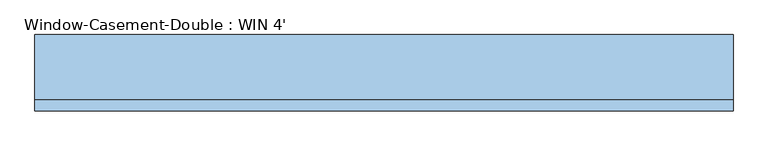
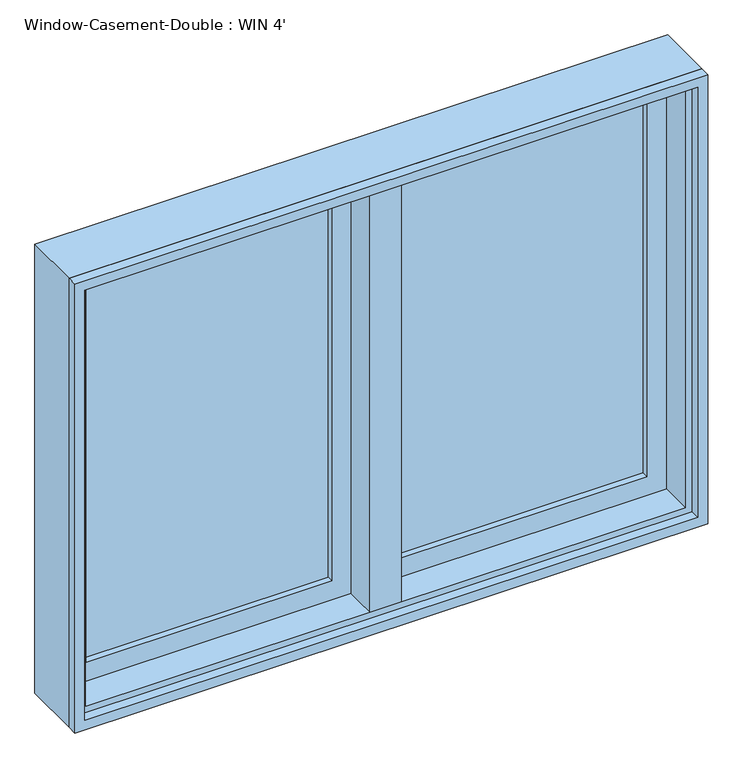
"""IFC4 building model written with IfcOpenShell, lengths in millimetres: window geometry, Window-Casement-Double : WIN 4'."""

from ifc_helpers import new_model, si_unit, frame, origin, place, context, project, spatial, polyline, outline, extrude, faceted_brep, source, transform, mapped, element, save


def window_casement_double_win_4_2967420f(model_context):
    return source(origin(), model_context, "Body", "SolidModel", [
        faceted_brep([(9.525, 76.2, 1816.1), (-9.525, 76.2, 1816.1), (-9.525, 25.4, 1816.1), (9.525, 25.4, 1816.1), (9.525, 76.2, 927.1), (9.525, 25.4, 927.1), (-9.525, 25.4, 927.1), (-9.525, 76.2, 927.1), (-9.525, 25.4, 946.15), (-9.525, 25.4, 1797.05), (-30.1625, 25.4, 946.15), (-30.1625, 25.4, 1797.05), (-30.1625, -38.1, 946.15), (-30.1625, -38.1, 1797.05), (30.1625, -38.1, 946.15), (30.1625, -38.1, 1797.05), (30.1625, 25.4, 946.15), (30.1625, 25.4, 1797.05), (9.525, 25.4, 946.15), (9.525, 25.4, 1797.05)], [[[0, 1, 2, 3]], [[4, 5, 6, 7]], [[1, 0, 4, 7]], [[2, 1, 7, 6, 8, 9]], [[9, 8, 10, 11]], [[11, 10, 12, 13]], [[13, 12, 14, 15]], [[15, 14, 16, 17]], [[17, 16, 18, 19]], [[0, 3, 19, 18, 5, 4]], [[18, 8, 6, 5]], [[9, 19, 3, 2]], [[8, 18, 16, 14, 12, 10]], [[19, 9, 11, 13, 15, 17]]]),
        extrude(outline(polyline([(-66.675, 57.15), (-66.675, 50.8), (-539.75, 50.8), (-539.75, 57.15), (-66.675, 57.15)])), frame((0.0, 0.0, 984.25), z_axis=(0.0, 0.0, 1.0), x_axis=(1.0, 0.0, 0.0)), (0.0, 0.0, 1.0), 774.7),
        extrude(outline(polyline([(-539.75, 38.1), (-539.75, 44.45), (-66.675, 44.45), (-66.675, 38.1), (-539.75, 38.1)])), frame((0.0, 0.0, 984.25), z_axis=(0.0, 0.0, 1.0), x_axis=(1.0, 0.0, 0.0)), (0.0, 0.0, 1.0), 774.7),
        extrude(outline(polyline([(539.75, 57.15), (539.75, 50.8), (66.675, 50.8), (66.675, 57.15), (539.75, 57.15)])), frame((0.0, 0.0, 984.25), z_axis=(0.0, 0.0, 1.0), x_axis=(1.0, 0.0, 0.0)), (0.0, 0.0, 1.0), 774.7),
        extrude(outline(polyline([(66.675, 38.1), (66.675, 44.45), (539.75, 44.45), (539.75, 38.1), (66.675, 38.1)])), frame((0.0, 0.0, 984.25), z_axis=(0.0, 0.0, 1.0), x_axis=(1.0, 0.0, 0.0)), (0.0, 0.0, 1.0), 774.7),
        extrude(outline(polyline([(1816.1, -596.9), (927.1, -596.9), (927.1, -9.525), (1816.1, -9.525), (1816.1, -596.9)]), holes=[polyline([(1758.95, -66.675), (984.25, -66.675), (984.25, -539.75), (1758.95, -539.75), (1758.95, -66.675)])]), frame((0.0, 25.4, 0.0), z_axis=(0.0, 1.0, 0.0), x_axis=(0.0, 0.0, 1.0)), (0.0, 0.0, 1.0), 44.45),
        extrude(outline(polyline([(927.1, 596.9), (1816.1, 596.9), (1816.1, 9.525), (927.1, 9.525), (927.1, 596.9)]), holes=[polyline([(984.25, 66.675), (1758.95, 66.675), (1758.95, 539.75), (984.25, 539.75), (984.25, 66.675)])]), frame((0.0, 25.4, 0.0), z_axis=(0.0, 1.0, 0.0), x_axis=(0.0, 0.0, 1.0)), (0.0, 0.0, 1.0), 44.45),
        extrude(outline(polyline([(1828.8, -609.6), (914.4, -609.6), (914.4, 609.6), (1828.8, 609.6), (1828.8, -609.6)]), holes=[polyline([(1809.75, 590.55), (933.45, 590.55), (933.45, -590.55), (1809.75, -590.55), (1809.75, 590.55)])]), frame((0.0, -57.15, 0.0), z_axis=(0.0, 1.0, 0.0), x_axis=(0.0, 0.0, 1.0)), (0.0, 0.0, 1.0), 19.05),
        faceted_brep([(577.85, 25.4, 1797.05), (577.85, -38.1, 1797.05), (-577.85, -38.1, 1797.05), (-577.85, 25.4, 1797.05), (596.9, 76.2, 1816.1), (596.9, 25.4, 1816.1), (-596.9, 25.4, 1816.1), (-596.9, 76.2, 1816.1), (609.6, -38.1, 1828.8), (609.6, 76.2, 1828.8), (-609.6, 76.2, 1828.8), (-609.6, -38.1, 1828.8), (-577.85, -38.1, 946.15), (-577.85, 25.4, 946.15), (-596.9, 25.4, 927.1), (-596.9, 76.2, 927.1), (-609.6, 76.2, 914.4), (-609.6, -38.1, 914.4), (577.85, -38.1, 946.15), (577.85, 25.4, 946.15), (596.9, 25.4, 927.1), (596.9, 76.2, 927.1), (609.6, 76.2, 914.4), (609.6, -38.1, 914.4)], [[[0, 1, 2, 3]], [[4, 5, 6, 7]], [[8, 9, 10, 11]], [[3, 2, 12, 13]], [[7, 6, 14, 15]], [[11, 10, 16, 17]], [[13, 12, 18, 19]], [[15, 14, 20, 21]], [[17, 16, 22, 23]], [[11, 17, 23, 8], [1, 18, 12, 2]], [[19, 18, 1, 0]], [[5, 20, 14, 6], [3, 13, 19, 0]], [[21, 20, 5, 4]], [[23, 22, 9, 8]], [[9, 22, 16, 10], [7, 15, 21, 4]]]),
    ])


if __name__ == "__main__":
    model = new_model("IFC4")
    model_context = context("Model", 3, world=origin())
    ifc_project = project(units=[si_unit("LENGTHUNIT", "METRE", prefix="MILLI")], contexts=[model_context])
    site = spatial("IfcSite", under=ifc_project)
    building = spatial("IfcBuilding", under=site)
    placement = place(None, origin())
    window_casement_double_win_4_shape = window_casement_double_win_4_2967420f(model_context)
    element("IfcWindow", 1, ObjectType="Window-Casement-Double : WIN 4'", at=placement, inside=building, context=model_context, shape_type="MappedRepresentation", body=[
        mapped(window_casement_double_win_4_shape, transform((0.0, 0.0, 0.0), x_axis=(1.0, 0.0, 0.0), y_axis=(0.0, 1.0, 0.0), z_axis=(0.0, 0.0, 1.0))),
    ])
    save(model, "model.ifc")

# Revit data of these elements
# Type "Window-Casement-Double : WIN 4'"
#   Type Mark = "18"
#   Fire Rating = "0.5h"
#   Assembly Code = "B2020100"
#   Analytic Construction = "Double glazing - domestic"
#   Frame Extension [instance default] = 0' - 0 1/4"
#   Window Inset [instance default] = 0' - 0"
#   Wall Thickness [instance default] = 0' - 6"
#   Interior Wall Closure [instance default] = 0' - 2 1/4"
#   Half Width = 2' - 0"
#   Visual Light Transmittance = 0.81
#   Thermal Resistance (R) = 1.8146 (h·ft²·°F)/BTU
#   Solar Heat Gain Coefficient = 0.76
#   Rough Width = 4' - 0 1/2"
#   Rough Height = 3' - 0 1/2"
#   Height = 3' - 0"
#   Heat Transfer Coefficient (U) = 0.5511 BTU/(h·ft²·°F)
#   Exterior Wall Closure [instance default] = 0' - 1 1/4"
#   Extension Jamb [instance default] = 0' - 2 1/4"
#   Default Sill Height = 3' - 0"
#   Width = 4' - 0"
#   Muntin Visibility = yes
#   Interior Trim Visibility [instance default] = yes
#   Exterior Trim Visibility [instance default] = yes
#   Extension Jamb Visibility [instance default] = yes
#   Interior Trim Material = Wood - Stained
#   Muntin Pattern = Muntin Pattern_2x2 : Muntin Pattern_2x2
#   Interior Trim = Trim-Window-Interior-Flat : Picture Frame
#   Interior Frame Material = Wood - Stained
#   Glass Panel Material = Glass
#   Exterior Trim Material = Clad - White
#   Exterior Trim = Trim-Window-Exterior-Flat : with Sill
#   Exterior Frame Material = Clad - White
#   Wall Closure = (empty or 0)
# Element 1 (IfcWindow, "Window-Casement-Double : WIN 4'")
#   Wall Thickness = 0' - 4 1/2"
#   Extension Jamb = 0' - 0 3/4"
#   Materials on its faces: "Wood - Stained", "Glass", "Clad - White"
# Materials
#   "Wood - Stained": class "Wood", colour RGB 224 178 126, transparency 0, Cost = 0
#   "Glass": class "Glass", colour RGB 0 128 192, transparency 0.75, Description = "Soda Lime Glass", Cost = 0
#   "Clad - White": class "Wood", colour RGB 242 242 238, transparency 0, Cost = 0
